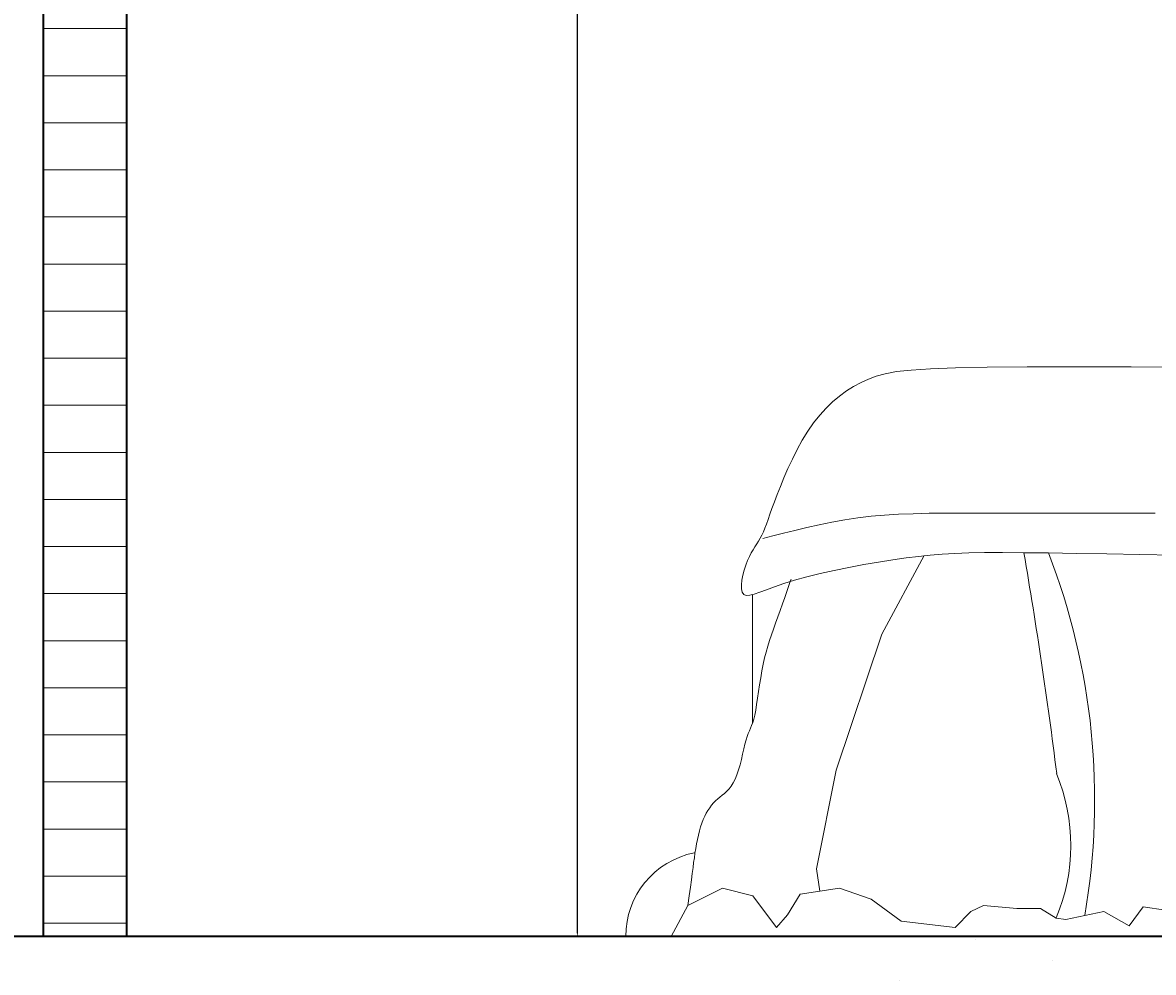
# Model space of a CAD drawing. Units: inches. Extents: x 2416 to 3391, y 1375 to 2496.
# Tile 9 of 13: x 3044 to 3105, y 2142 to 2193. Entities that reach past the tile are written whole.
import ezdxf

# ---------------------------------------------------------------- set-up
doc = ezdxf.new("R2010")
doc.units = ezdxf.units.IN
for name, color, linetype, lineweight in [('A-ANNO-DIMS', 2, 'Continuous', 18), ('A-FLOR-PATT', 252, 'Continuous', 13), ('A-FURN', 8, 'Continuous', 18), ('A-SECT', 7, 'Continuous', 35), ('A-WALL-PATT', 252, 'Continuous', 13)]:
    doc.layers.add(name, color=color, linetype=linetype, lineweight=lineweight)
doc.styles.get("Standard").update_dxf_attribs({"font": 'arial.ttf'})
doc.dimstyles.get("Standard").update_dxf_attribs({"dimtxt": 0.18, "dimasz": 0.18, "dimexe": 0.18, "dimexo": 0.0625, "dimgap": 0.09, "dimtad": 0, "dimtih": 1, "dimtoh": 1, "dimdec": 4, "dimzin": 0, "dimdsep": 46, "dimtxsty": 'Standard', "dimcen": 0.09, "dimadec": 0, "dimazin": 0, "dimtfac": 1, "dimtdec": 4, "dimtofl": 0, "dimtmove": 0, "dimatfit": 3, "dimfxl": 1, "dimtolj": 1, "dimtzin": 0, "dimarcsym": 0})

# ---------------------------------------------------------------- blocks, each defined once
blk = doc.blocks.new('A$C08BC4B9A')
for p, q in [((1640.5, 563.3), (1579.1, 563)), ((1695.8, 563.4), (1640.5, 563.3)), ((1743.5, 563.3), (1695.8, 563.4)), ((1782.8, 563), (1743.5, 563.3)), ((1814.2, 562.4), (1782.8, 563)), ((1838.9, 561.5), (1814.2, 562.4)), ((1858, 560.2), (1838.9, 561.5)), ((1872.6, 558.6), (1858, 560.2)), ((1883.7, 556.6), (1872.6, 558.6)), ((1892.6, 554.2), (1883.7, 556.6)), ((1900.3, 551.3), (1892.6, 554.2)), ((1907.7, 547.9), (1900.3, 551.3)), ((1915, 544), (1907.7, 547.9)), ((1922.1, 539.6), (1915, 544)), ((1929, 534.5), (1922.1, 539.6)), ((1935.8, 528.9), (1929, 534.5)), ((1942.3, 522.6), (1935.8, 528.9)), ((1948.6, 515.6), (1942.3, 522.6)), ((1954.6, 508), (1948.6, 515.6)), ((1960.4, 499.6), (1954.6, 508)), ((1965.8, 490.7), (1960.4, 499.6)), ((1970.9, 481.5), (1965.8, 490.7)), ((1975.6, 472.1), (1970.9, 481.5)), ((1980, 462.7), (1975.6, 472.1)), ((1984, 453.6), (1980, 462.7)), ((1987.5, 445), (1984, 453.6)), ((1990.7, 437), (1987.5, 445)), ((1993.4, 429.7), (1990.7, 437)), ((1995.8, 423.3), (1993.4, 429.7)), ((1616.7, 418.7), (1649.3, 418.7)), ((1649.3, 418.7), (1680.1, 418.7)), ((1680.1, 418.7), (1709, 418.7)), ((1709, 418.7), (1736, 418.7)), ((1736, 418.7), (1760.9, 418.7)), ((1760.9, 418.7), (1783.8, 418.7)), ((1783.8, 418.7), (1804.5, 418.7)), ((1804.5, 418.7), (1823.2, 418.6)), ((1823.2, 418.6), (1840.3, 418.5)), ((1840.3, 418.5), (1856.1, 418.1)), ((1856.1, 418.1), (1870.7, 417.6)), ((1870.7, 417.6), (1884.5, 416.7)), ((1884.5, 416.7), (1897.8, 415.6)), ((1897.8, 415.6), (1910.8, 414)), ((1910.8, 414), (1923.7, 412)), ((1997.8, 417.5), (1995.8, 423.3)), ((1999.6, 412.4), (1997.8, 417.5)), ((1923.7, 412), (1936.5, 409.7)), ((1936.5, 409.7), (1949.1, 407.1)), ((1949.1, 407.1), (1961.3, 404.4)), ((1961.3, 404.4), (1973.1, 401.6)), ((2001.3, 407.8), (1999.6, 412.4)), ((2002.8, 403.7), (2001.3, 407.8)), ((2004.3, 400.1), (2002.8, 403.7)), ((1973.1, 401.6), (1984.4, 398.8)), ((1984.4, 398.8), (1995, 396.1)), ((1995, 396.1), (2004.8, 393.6)), ((2005.8, 396.8), (2004.3, 400.1)), ((2007.5, 393.8), (2005.8, 396.8)), ((2009.2, 390.9), (2007.5, 393.8)), ((2010.9, 388.2), (2009.2, 390.9)), ((2012.7, 385.4), (2010.9, 388.2)), ((2014.5, 382.5), (2012.7, 385.4)), ((2016.4, 379.3), (2014.5, 382.5)), ((1597.9, 377.2), (1632, 377.8)), ((1632, 377.8), (1664.4, 378.4)), ((1664.4, 378.4), (1694.6, 378.9)), ((1694.6, 378.9), (1722.2, 379.3)), ((1722.2, 379.3), (1746.7, 379.5)), ((1746.7, 379.5), (1767.7, 379.7)), ((1767.7, 379.7), (1785.7, 379.6)), ((1785.7, 379.6), (1801.2, 379.4)), ((1801.2, 379.4), (1814.9, 378.9)), ((1814.9, 378.9), (1827.4, 378.2)), ((1827.4, 378.2), (1839.2, 377.2)), ((1839.2, 377.2), (1850.9, 375.9)), ((1845.1, 376.6), (1887, 298.9)), ((1850.9, 375.9), (1863.2, 374.3)), ((1863.2, 374.3), (1876.4, 372.4)), ((1876.4, 372.4), (1890.5, 370.2)), ((1890.5, 370.2), (1905, 367.7)), ((2018.2, 375.7), (2016.4, 379.3)), ((2020, 371.7), (2018.2, 375.7)), ((2021.7, 367.2), (2020, 371.7)), ((1905, 367.7), (1919.7, 364.9)), ((1919.7, 364.9), (1934.2, 362)), ((1934.2, 362), (1948.2, 358.9)), ((1948.2, 358.9), (1961.4, 355.7)), ((2023.2, 362.2), (2021.7, 367.2)), ((2024.6, 357.2), (2023.2, 362.2)), ((1961.4, 355.7), (1973.5, 352.4)), ((1973.5, 352.4), (1984.1, 349.1)), ((1977.1, 352.6), (1976.8, 353.5)), ((1978, 350), (1977.1, 352.6)), ((1979.4, 346.1), (1978, 350)), ((1984.1, 349.1), (1993.3, 345.9)), ((2025.5, 352.3), (2024.6, 357.2)), ((2026, 347.7), (2025.5, 352.3)), ((2025.9, 343.7), (2026, 347.7)), ((1981.2, 341.1), (1979.4, 346.1)), ((1983.2, 335.3), (1981.2, 341.1)), ((1993.3, 345.9), (2001.3, 342.9)), ((2001.3, 342.9), (2007.9, 340.5)), ((2007.9, 340.5), (2013.4, 338.6)), ((2013.4, 338.6), (2017.8, 337.5)), ((2015, 211.3), (2015, 338.2)), ((2017.8, 337.5), (2021.2, 337.3)), ((2021.2, 337.3), (2023.6, 338.3)), ((2023.6, 338.3), (2025.2, 340.5)), ((2025.2, 340.5), (2025.9, 343.7)), ((1985.5, 329), (1983.2, 335.3)), ((1987.8, 322.5), (1985.5, 329)), ((1990.1, 316.1), (1987.8, 322.5)), ((1992.3, 309.9), (1990.1, 316.1)), ((1994.4, 304), (1992.3, 309.9)), ((1996.4, 298.3), (1994.4, 304)), ((1887, 298.9), (1932.4, 164.5)), ((1998.2, 292.7), (1996.4, 298.3)), ((2000, 287.1), (1998.2, 292.7)), ((2001.6, 281.3), (2000, 287.1)), ((2003.1, 275.4), (2001.6, 281.3)), ((2004.5, 269.2), (2003.1, 275.4)), ((2005.8, 262.6), (2004.5, 269.2)), ((2006.9, 255.8), (2005.8, 262.6)), ((2008, 248.9), (2006.9, 255.8)), ((2009, 242.1), (2008, 248.9)), ((2010, 235.6), (2009, 242.1)), ((2011, 229.5), (2010, 235.6)), ((2011.9, 223.9), (2011, 229.5)), ((2012.9, 219), (2011.9, 223.9)), ((2013.9, 215), (2012.9, 219)), ((2014.9, 211.6), (2013.9, 215)), ((2015.9, 208.7), (2014.9, 211.6)), ((2017, 206), (2015.9, 208.7)), ((2018.1, 203.5), (2017, 206)), ((2019.2, 200.8), (2018.1, 203.5)), ((2020.3, 197.8), (2019.2, 200.8)), ((2021.4, 194.3), (2020.3, 197.8)), ((2022.5, 190.2), (2021.4, 194.3)), ((2023.7, 185.5), (2022.5, 190.2)), ((2024.9, 180.4), (2023.7, 185.5)), ((2026.1, 175.1), (2024.9, 180.4)), ((2027.4, 169.8), (2026.1, 175.1)), ((2028.9, 164.7), (2027.4, 169.8)), ((1932.4, 164.5), (1951.6, 66.8)), ((2030.5, 159.8), (2028.9, 164.7)), ((2032.2, 155.5), (2030.5, 159.8)), ((2034.1, 151.8), (2032.2, 155.5)), ((2036.1, 148.6), (2034.1, 151.8)), ((2038.3, 145.9), (2036.1, 148.6)), ((2040.5, 143.6), (2038.3, 145.9)), ((2042.8, 141.5), (2040.5, 143.6)), ((2045, 139.6), (2042.8, 141.5)), ((2047.3, 137.8), (2045, 139.6)), ((2049.5, 136), (2047.3, 137.8)), ((2051.6, 134.1), (2049.5, 136)), ((2053.6, 132), (2051.6, 134.1)), ((2055.6, 129.7), (2053.6, 132)), ((2057.4, 127.3), (2055.6, 129.7)), ((2059.1, 124.7), (2057.4, 127.3)), ((2060.8, 121.9), (2059.1, 124.7)), ((2062.3, 118.9), (2060.8, 121.9)), ((2063.8, 115.6), (2062.3, 118.9)), ((2065.1, 112), (2063.8, 115.6)), ((2066.4, 108.3), (2065.1, 112)), ((2067.5, 104.3), (2066.4, 108.3)), ((2068.6, 100.2), (2067.5, 104.3)), ((2069.5, 95.9), (2068.6, 100.2)), ((2070.4, 91.5), (2069.5, 95.9)), ((2071.2, 87), (2070.4, 91.5)), ((2072, 82.5), (2071.2, 87)), ((2072.6, 77.9), (2072, 82.5)), ((2073.3, 73.2), (2072.6, 77.9)), ((2073.9, 68.1), (2073.3, 73.2)), ((2074.7, 62.4), (2073.9, 68.1)), ((1951.6, 66.8), (1948.4, 44.8)), ((2075.5, 56), (2074.7, 62.4)), ((2076.5, 48.7), (2075.5, 56)), ((1897.6, 37), (1928.9, 47.9)), ((1928.9, 47.9), (1968, 41.7)), ((2014.9, 40.1), (2044.6, 47.9)), ((2044.6, 47.9), (2079, 30.7)), ((2077.6, 40.3), (2076.5, 48.7)), ((1867.9, 15.1), (1897.6, 37)), ((1968, 41.7), (1980.5, 21.4)), ((1991.4, 8.9), (2014.9, 40.1)), ((2079, 30.7), (2077.6, 40.3)), ((1606.6, 26.1), (1628.5, 29.2)), ((1628.5, 29.2), (1642.6, 10.4)), ((1642.6, 10.4), (1667.6, 24.5)), ((1667.6, 24.5), (1705.2, 16.7)), ((1714.5, 18.2), (1730.2, 27.6)), ((1730.2, 27.6), (1745.8, 27.6)), ((1745.8, 27.6), (1753.7, 27.6)), ((1753.7, 27.6), (1786.5, 30.7)), ((1786.5, 30.7), (1799, 24.5)), ((1799, 24.5), (1814.7, 8.9)), ((2079, 30.7), (2095.6, 0)), ((1705.2, 16.7), (1714.5, 18.2)), ((1814.7, 8.9), (1867.9, 15.1)), ((1980.5, 21.4), (1991.4, 8.9)), ((0, 0), (2150.5, 0))]:
    blk.add_line(p, q)
for centre, radius, start, end in [((2353.4, 135.1), 676.8, 158.8487, 189.7401), ((6455, -433.2), 4778, 170.2062, 172.8555), ((1887.2, 90.1), 187, 157.7155, 202.6016), ((2056.3, 0.1), 84.2, 359.9053, 78.7345)]:
    blk.add_arc(centre, radius, start, end)
blk = doc.blocks.new('*D86')
at = {"layer": 'A-ANNO-DIMS', "color": 0, "lineweight": -2, "transparency": 16777216}
for p, q in [((3049.755, 2263.861), (3074.272, 2263.861)), ((3074.092, 2263.681), (3074.092, 2204.043)), ((3074.092, 2144.041), (3074.092, 2203.679)), ((3049.755, 2143.861), (3074.272, 2143.861))]:
    blk.add_line(p, q, dxfattribs=at)
at = {"layer": 'A-ANNO-DIMS', "color": 0, "transparency": 16777216}
for points in [[(3074.062, 2263.681), (3074.122, 2263.681), (3074.092, 2263.861)], [(3074.062, 2144.041), (3074.122, 2144.041), (3074.092, 2143.861)]]:
    blk.add_solid(points, dxfattribs=at)
at = {"layer": 'Defpoints', "color": 0, "transparency": 16777216}
for p in [(3049.692, 2263.861), (3049.692, 2143.861), (3074.092, 2143.861)]:
    blk.add_point(p, dxfattribs=at)
at = {"layer": 'A-ANNO-DIMS', "color": 0, "transparency": 16777216, "insert": (3074.092, 2203.861), "char_height": 0.18, "attachment_point": 5}
blk.add_mtext('\\A1;120', dxfattribs=at)

msp = doc.modelspace()

# ---------------------------------------------------------------- hatches: boundary and pattern name
at = {"layer": 'A-FLOR-PATT'}
h = msp.add_hatch(dxfattribs=at)
h.set_pattern_fill('AR-CONC', color=256, scale=0.13, style=0)
h.paths.add_polyline_path([(2904.1924, 2125.8608), (3202.6924, 2125.8608), (3202.6924, 2143.8608), (2904.1924, 2143.8608)])
at = {"layer": 'A-WALL-PATT'}
h = msp.add_hatch(dxfattribs=at)
h.set_pattern_fill('ANSI31', color=256, scale=0.802205, angle=-45, style=0)
h.paths.add_polyline_path([(3045.1924, 2143.8608), (3049.6924, 2143.8608), (3049.6924, 2263.8608), (3045.1924, 2263.8608)])

# ---------------------------------------------------------------- linework, layer by layer
at = {"layer": 'A-SECT'}
for p, q in [((3045.1924, 2263.8608), (3045.1924, 2143.8608)), ((3049.6924, 2263.8608), (3049.6924, 2143.8608)), ((3202.6924, 2143.8608), (2904.1924, 2143.8608))]:
    msp.add_line(p, q, dxfattribs=at)

# ---------------------------------------------------------------- block references
at = {"layer": 'A-FURN', "xscale": -0.0546942147408242, "yscale": 0.0546942147408242, "zscale": 0.0546942147408242}
msp.add_blockref('A$C08BC4B9A', (3193.7816, 2143.8608), dxfattribs=at)

# ---------------------------------------------------------------- dimensions: what is measured, and where the dimension line sits
at = {"layer": 'A-ANNO-DIMS'}
dim = msp.add_linear_dim(base=(3074.0924, 2143.8608), p1=(3049.6924, 2263.8608), p2=(3049.6924, 2143.8608), angle=270, dimstyle='Standard', override={"dimdec": 0, "dimlfac": 1, "dimrnd": 0, "dimzin": 0, "dimdsep": 46, "dimlunit": 2}, dxfattribs=at)
dim.commit()
dim.dimension.update_dxf_attribs({"geometry": '*D86', "text_midpoint": (3074.0924, 2203.8608)})

doc.saveas('drawing.dxf')
